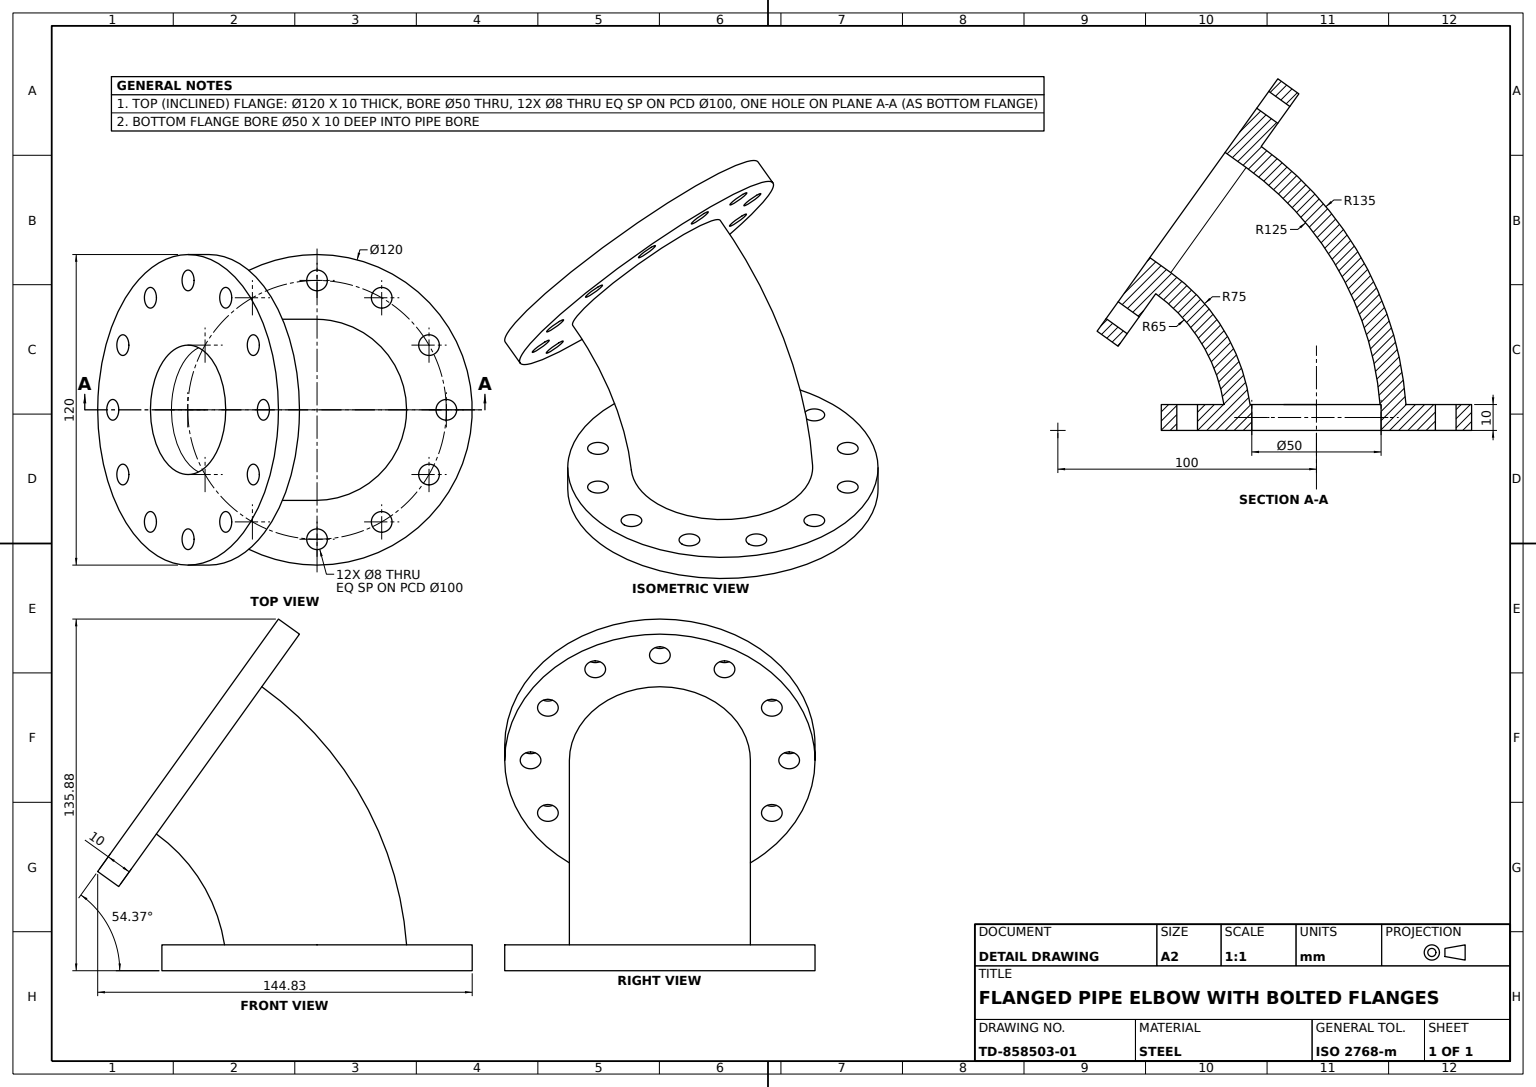
from build123d import *

# Parameters (mm, degrees)
BOTTOM_FLANGE_PROFILE_R            = 60
BOTTOM_FLANGE_120_DEPTH            = 10
ELBOW_PIPE_SWEEP_PROFILE_R         = 35
ELBOW_PIPE_SWEEP_PROFILE_R_2       = 25
TOP_FLANGE_PROFILE_R               = 60
TOP_FLANGE_120_DEPTH               = 10
TOP_BORE_PROFILE_A_R               = 25
TOP_FLANGE_BORE_CUT_A_DEPTH        = 5
TOP_BORE_PROFILE_B_R               = 25
TOP_FLANGE_BORE_CUT_B_DEPTH        = 5
BOTTOM_BORE_PROFILE_R              = 25
BOTTOM_FLANGE_BORE_DEPTH           = 10
TOP_BOLT_HOLE_CIRCLE_R             = 4
TOP_FLANGE_BOLT_HOLES_12X_DEPTH    = 10
BOTTOM_BOLT_HOLE_CIRCLE_R          = 4
BOTTOM_FLANGE_BOLT_HOLES_12X_DEPTH = 10


with BuildPart() as part:
    # Bottom Flange Profile → Bottom Flange _120 (new body)
    with BuildSketch(Plane(origin=(0, 0, 0), x_dir=(1, 0, 0), z_dir=(0, 1, 0))):
        with Locations(Location((0, 0, 0), (0, 0, 270))):
            Circle(BOTTOM_FLANGE_PROFILE_R)
    extrude(amount=BOTTOM_FLANGE_120_DEPTH)

    # Elbow Pipe Sweep: sweep along a path in Elbow Bend Path
    with BuildLine(Plane.XY) as elbow_pipe_sweep_path:
        ThreePointArc((0, 0), (-11.047311529, 45.688283112), (-41.748384274, 81.281912289))
    # Elbow Pipe Sweep profile (on start of the path) → Elbow Pipe Sweep (sweep)
    with BuildSketch(Plane(origin=(0, 0, 0), x_dir=(1, 0, 0), z_dir=(0, 1, 0))):
        Circle(ELBOW_PIPE_SWEEP_PROFILE_R)
        Circle(ELBOW_PIPE_SWEEP_PROFILE_R_2, mode=Mode.SUBTRACT)
    sweep(path=elbow_pipe_sweep_path.line)

    # Top Flange Profile → Top Flange _120 (add)
    with BuildSketch(Plane(origin=(-66.067492653, 47.348027201, 0), x_dir=(0, 0, 1), z_dir=(-0.8128191228882113, 0.5825161572585252, 0))):
        with Locations(Location((0, 41.748384274, 0), (0, 0, 270))):
            Circle(TOP_FLANGE_PROFILE_R)
    extrude(amount=TOP_FLANGE_120_DEPTH)

    # Top Bore Profile A → Top Flange Bore Cut A (cut)
    with BuildSketch(Plane(origin=(-74.195683882, 53.173188774, 0), x_dir=(0, 0, 1), z_dir=(-0.8128191228882113, 0.5825161572585252, 0))):
        with Locations(Location((0, 41.748384274, 0), (0, 0, 270))):
            Circle(TOP_BORE_PROFILE_A_R)
    extrude(amount=-TOP_FLANGE_BORE_CUT_A_DEPTH, mode=Mode.SUBTRACT)

    # Top Bore Profile B → Top Flange Bore Cut B (cut)
    with BuildSketch(Plane(origin=(-70.131588268, 50.260607987, 0), x_dir=(0, 0, 1), z_dir=(-0.8128191228882113, 0.5825161572585252, 0))):
        with Locations(Location((0, 41.748384274, 0), (0, 0, 270))):
            Circle(TOP_BORE_PROFILE_B_R)
    extrude(amount=-TOP_FLANGE_BORE_CUT_B_DEPTH, mode=Mode.SUBTRACT)

    # Bottom Bore Profile → Bottom Flange Bore (cut)
    with BuildSketch(Plane.XZ):
        with Locations(Location((0, 0, 0), (0, 0, 270))):
            Circle(BOTTOM_BORE_PROFILE_R)
    extrude(amount=-BOTTOM_FLANGE_BORE_DEPTH, mode=Mode.SUBTRACT)

    # Top Bolt Hole Circle → Top Flange Bolt Holes 12x (cut)
    with BuildSketch(Plane(origin=(-74.195683882, 53.173188774, 0), x_dir=(0, 0, 1), z_dir=(-0.8128191228882113, 0.5825161572585252, 0))):
        with Locations(Location((0, 91.748384274, 0), (0, 0, 270))):
            Circle(TOP_BOLT_HOLE_CIRCLE_R)
        with Locations(Location((25, 85.049654463, 0), (0, 0, 270))):
            Circle(TOP_BOLT_HOLE_CIRCLE_R)
        with Locations(Location((43.301270189, 66.748384274, 0), (0, 0, 270))):
            Circle(TOP_BOLT_HOLE_CIRCLE_R)
        with Locations(Location((50, 41.748384274, 0), (0, 0, 270))):
            Circle(TOP_BOLT_HOLE_CIRCLE_R)
        with Locations(Location((43.301270189, 16.748384274, 0), (0, 0, 270))):
            Circle(TOP_BOLT_HOLE_CIRCLE_R)
        with Locations(Location((25, -1.552885915, 0), (0, 0, 270))):
            Circle(TOP_BOLT_HOLE_CIRCLE_R)
        with Locations(Location((0, -8.251615726, 0), (0, 0, 270))):
            Circle(TOP_BOLT_HOLE_CIRCLE_R)
        with Locations(Location((-25, -1.552885915, 0), (0, 0, 270))):
            Circle(TOP_BOLT_HOLE_CIRCLE_R)
        with Locations(Location((-43.301270189, 16.748384274, 0), (0, 0, 270))):
            Circle(TOP_BOLT_HOLE_CIRCLE_R)
        with Locations(Location((-50, 41.748384274, 0), (0, 0, 270))):
            Circle(TOP_BOLT_HOLE_CIRCLE_R)
        with Locations(Location((-43.301270189, 66.748384274, 0), (0, 0, 270))):
            Circle(TOP_BOLT_HOLE_CIRCLE_R)
        with Locations(Location((-25, 85.049654463, 0), (0, 0, 270))):
            Circle(TOP_BOLT_HOLE_CIRCLE_R)
    extrude(amount=-TOP_FLANGE_BOLT_HOLES_12X_DEPTH, mode=Mode.SUBTRACT)

    # Bottom Bolt Hole Circle → Bottom Flange Bolt Holes 12x (cut)
    with BuildSketch(Plane.XZ):
        with Locations(Location((0, 50, 0), (0, 0, 270))):
            Circle(BOTTOM_BOLT_HOLE_CIRCLE_R)
        with Locations(Location((25, 43.301270189, 0), (0, 0, 270))):
            Circle(BOTTOM_BOLT_HOLE_CIRCLE_R)
        with Locations(Location((43.301270189, 25, 0), (0, 0, 270))):
            Circle(BOTTOM_BOLT_HOLE_CIRCLE_R)
        with Locations(Location((50, 0, 0), (0, 0, 270))):
            Circle(BOTTOM_BOLT_HOLE_CIRCLE_R)
        with Locations(Location((43.301270189, -25, 0), (0, 0, 270))):
            Circle(BOTTOM_BOLT_HOLE_CIRCLE_R)
        with Locations(Location((25, -43.301270189, 0), (0, 0, 270))):
            Circle(BOTTOM_BOLT_HOLE_CIRCLE_R)
        with Locations(Location((0, -50, 0), (0, 0, 270))):
            Circle(BOTTOM_BOLT_HOLE_CIRCLE_R)
        with Locations(Location((-25, -43.301270189, 0), (0, 0, 270))):
            Circle(BOTTOM_BOLT_HOLE_CIRCLE_R)
        with Locations(Location((-43.301270189, -25, 0), (0, 0, 270))):
            Circle(BOTTOM_BOLT_HOLE_CIRCLE_R)
        with Locations(Location((-50, 0, 0), (0, 0, 270))):
            Circle(BOTTOM_BOLT_HOLE_CIRCLE_R)
        with Locations(Location((-43.301270189, 25, 0), (0, 0, 270))):
            Circle(BOTTOM_BOLT_HOLE_CIRCLE_R)
        with Locations(Location((-25, 43.301270189, 0), (0, 0, 270))):
            Circle(BOTTOM_BOLT_HOLE_CIRCLE_R)
    extrude(amount=-BOTTOM_FLANGE_BOLT_HOLES_12X_DEPTH, mode=Mode.SUBTRACT)


solid = part.part
